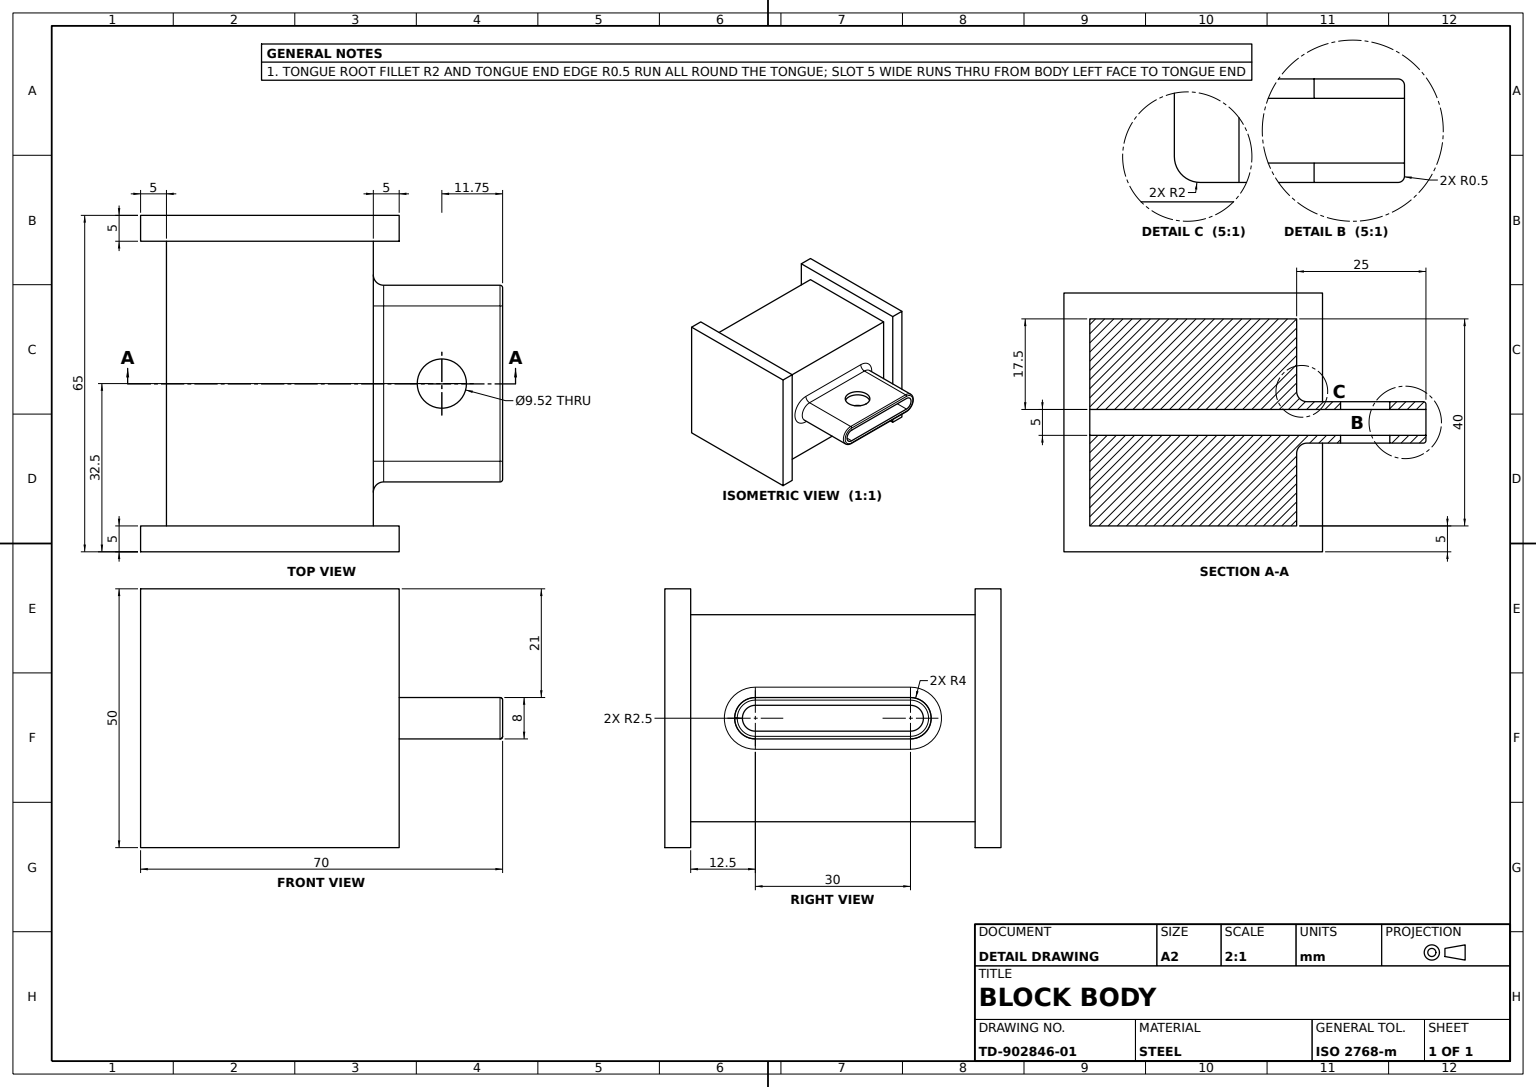
SolidWorks part; units mm, degrees
material "Plain Carbon Steel"
ref_plane "Front Plane" through (0, 0, 0) normal (0, 0, 1) x (1, 0, 0)
ref_plane "Top Plane" through (0, 0, 0) normal (0, 1, 0) x (1, 0, 0)
ref_plane "Right Plane" through (0, 0, 0) normal (1, 0, 0) x (0, 0, -1)
sketch "Front Flange Sketch" plane through (0, 0, 0) normal (0, 0, 1) x (1, 0, 0)
  line L0 (0, 0) -> (0, 50)
  line L1 (0, 50) -> (50, 50)
  line L2 (50, 50) -> (50, 0)
  line L3 (50, 0) -> (0, 0)
  dimension "D1" = 50
  dimension "D2" = 50
extrude "Front Flange 50x50x5" add sketch "Front Flange Sketch" along normal blind 5
sketch "Body Block Sketch" plane through (0, 0, 5) normal (0, 0, 1) x (1, 0, 0)
  line L0 (0, 0) -> (50, 0) construction
  line L1 (5, 45) -> (45, 45)
  line L2 (5, 45) -> (5, 5)
  line L3 (5, 5) -> (45, 5)
  line L4 (45, 45) -> (45, 5)
  line L5 (0, 50) -> (0, 0) construction
  dimension "D1" = 40
  dimension "D2" = 40
  dimension "D3" = 5
  dimension "D4" = 5
extrude "Body Block 40x40x55" add sketch "Body Block Sketch" along normal blind 55
sketch "Rear Flange Sketch" plane through (0, 0, 60) normal (0, 0, 1) x (1, 0, 0)
  line L0 (0, 50) -> (50, 50)
  line L1 (50, 50) -> (50, 0)
  line L2 (50, 0) -> (0, 0)
  line L3 (0, 0) -> (0, 50)
extrude "Rear Flange 5mm" add sketch "Rear Flange Sketch" along normal blind 5
sketch "Tongue Profile Sketch" plane through (45, 0, 0) normal (1, 0, 0) x (0, 0, -1)
  line L0 (-5, 25) -> (-60, 25)
  line L1 (-5, 0) -> (-5, 50) construction
  line L2 (-60, 5) -> (-60, 45) construction
  line L3 (-47.5, 29) -> (-17.5, 29)
  line L4 (-47.5, 21) -> (-17.5, 21)
  arc A0 (-47.5, 29) -> (-47.5, 21) centre (-47.5, 25) ccw
  arc A1 (-17.5, 21) -> (-17.5, 29) centre (-17.5, 25) ccw
  dimension "D3" = 8
  dimension "D4" = 8
  dimension "D1" = 30
  dimension "D2" = 12.5
  dimension "D5" = 30
  dimension "D6" = 30
extrude "Obround Tongue" add sketch "Tongue Profile Sketch" along normal blind 25 contours L4 A1 L0 A0
sketch "Tongue Slot Sketch" plane through (70, 0, 0) normal (1, 0, 0) x (0, 0, -1)
  line L0 (-47.5, 22.5) -> (-17.5, 22.5)
  line L1 (-17.5, 27.5) -> (-47.5, 27.5)
  arc A0 (-47.5, 27.5) -> (-47.5, 22.5) centre (-47.5, 25) ccw
  arc A1 (-17.5, 22.5) -> (-17.5, 27.5) centre (-17.5, 25) ccw
  dimension "D1" = 5
  dimension "D2" = 5
  dimension "D3" = 30
  dimension "D4" = 30
extrude "Tongue Slot Cut" cut sketch "Tongue Slot Sketch" against normal through all
fillet "Tongue Root Fillet R2" radius 2 4 edges at (45, 25, 51.5) (45, 21, 32.5) (45, 25, 13.5) (45, 29, 32.5)
fillet "Tongue Edge Fillet R0.5" radius 0.5 4 edges at (70, 25, 51.5) (70, 21, 32.5) (70, 25, 13.5) (70, 29, 32.5)
sketch "Tongue Hole Sketch" plane through (0, 21, 0) normal (0, -1, 0) x (1, 0, 0)
  line L0 (69.5, 17.5) -> (47, 17.5) construction
  line L3 (69.5, 17.5) -> (69.5, 47.5) construction
  circle A0 centre (58.25, 32.5) radius 4.7595
  dimension "D1" = 9.519
  dimension "D2" = 15
  dimension "D3" = 11.25
extrude "Tongue Cross Hole" cut sketch "Tongue Hole Sketch" against normal through all
